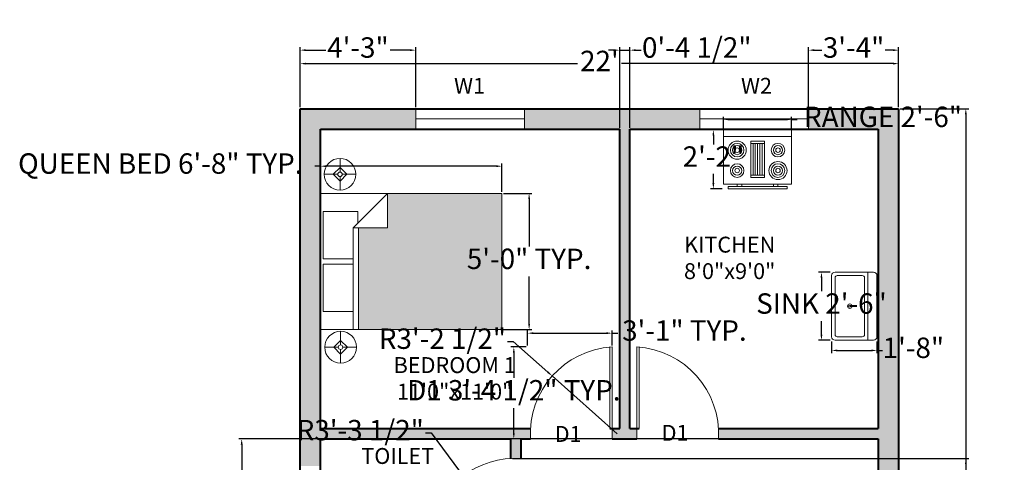
# Model space of a CAD drawing. Units: inches. Extents: x 1883 to 2353, y 1976 to 2541.
# Tile 5 of 5: x 1883 to 2317, y 2346 to 2541. Entities that reach past the tile are written whole.
import ezdxf

# ---------------------------------------------------------------- set-up
doc = ezdxf.new("R2010")
doc.units = ezdxf.units.IN
for name, color, linetype, lineweight in [('A-ANNO-DIMS', 2, 'Continuous', 18), ('A-ANNO-TEXT', 7, 'Continuous', 18), ('A-AREA-IDEN', 7, 'Continuous', 18), ('A-DOOR', 3, 'Continuous', 18), ('A-EQPM', 8, 'Continuous', 18), ('A-FLOR-FIXT', 9, 'Continuous', 18), ('A-FURN', 8, 'Continuous', 18), ('A-GLAZ', 4, 'Continuous', 18), ('A-WALL', 7, 'Continuous', 40)]:
    doc.layers.add(name, color=color, linetype=linetype, lineweight=lineweight)
doc.layers.add('A-FURN-PATT', color=18, linetype='Continuous', lineweight=13, true_color=0x000000)
doc.layers.add('A-WALL-PATT', color=67, linetype='Continuous', lineweight=13, true_color=0x727430)
doc.styles.get("Standard").update_dxf_attribs({"font": 'arial.ttf'})
doc.dimstyles.new('ISO-25', dxfattribs={"dimtxt": 9, "dimasz": 2.5, "dimexe": 1.25, "dimexo": 0.625, "dimgap": 2, "dimtad": 0, "dimtih": 1, "dimtoh": 1, "dimdec": 1, "dimlunit": 4, "dimtxsty": 'Standard', "dimcen": 2.5, "dimadec": 0, "dimazin": 0, "dimtfac": 1, "dimtdec": 1, "dimtmove": 0, "dimatfit": 3, "dimfxl": 1, "dimarcsym": 0})

# ---------------------------------------------------------------- blocks, each defined once
blk = doc.blocks.new('Bed - Queen')
for p, q in [((0, -80.00003), (0, 0)), ((0, 0), (59.99999, 0)), ((59.99999, 0), (59.99999, -80.00003)), ((7.99999, -1.2), (28.79998, -1.2)), ((7.99999, -14.4), (7.99999, -1.2)), ((28.79998, -1.2), (28.79998, -14.4)), ((31.19999, -1.2), (51.99999, -1.2)), ((31.19999, -14.4), (31.19999, -1.2)), ((51.99999, -1.2), (51.99999, -16.4)), ((0, -14.4), (44.8, -14.4)), ((44.8, -16.8), (0, -16.8)), ((59.99999, -29.6), (44.8, -14.4)), ((44.8, -14.4), (44.8, -29.6)), ((51.99999, -16.4), (46.79936, -16.4)), ((44.8, -29.6), (59.99999, -29.6)), ((59.99999, -80.00003), (0, -80.00003))]:
    blk.add_line(p, q)
blk = doc.blocks.new('Range-Oven - 30 in top')
for p, q in [((0, -3), (30, -3)), ((12, -6), (18, -6)), ((13, -20), (13, -6)), ((14, -6), (14, -20)), ((15, -20), (15, -6)), ((16, -6), (16, -20)), ((17, -20), (17, -6)), ((18, -20), (12, -20)), ((6, -24), (6, -25)), ((8, -25), (8, -24)), ((22, -25), (22, -24)), ((24, -24), (24, -25))]:
    blk.add_line(p, q)
for points in [[(0, -24), (0, 0), (30, 0), (30, -24)], [(12, -21), (12, -5), (18, -5), (18, -21)], [(2, -26), (2, -25), (28, -25), (28, -26)]]:
    blk.add_lwpolyline(points, close=True)
for centre, radius in [((6, -9), 4), ((6, -9), 3), ((6, -9), 2), ((6, -9), 1), ((24, -9), 3), ((24, -9), 2), ((24, -9), 1), ((6, -18), 3), ((6, -18), 2), ((6, -18), 1), ((24, -18), 4), ((24, -18), 3), ((24, -18), 2), ((24, -18), 1)]:
    blk.add_circle(centre, radius)
blk = doc.blocks.new('Sink-single - 30 in top')
blk.add_line((-15, -3.999996), (15, -3.999996))
for points in [[(-13.5, 0), (13.5, 0)], [(-15, -18.499996), (-15, -1.5)], [(15, -1.5), (15, -18.499996)], [(-13.5, -17.499996), (-13.5, -6.499996)], [(-12.5, -5.499996), (12.5, -5.499996)], [(13.5, -6.499996), (13.5, -17.499996)], [(13.5, -19.999996), (-13.5, -19.999996)], [(12.5, -18.499996), (-12.5, -18.499996)]]:
    blk.add_lwpolyline(points)
for radius in [1, 0.5]:
    blk.add_circle((0, -11.999996), radius)
for centre, radius, start, end in [((-13.5, -1.5), 1.5, 90, 180), ((13.5, -1.5), 1.5, 0, 90), ((-12.5, -6.499996), 1, 90, 180), ((12.5, -6.499996), 1, 0, 90), ((-13.5, -18.499996), 1.5, 180, 270), ((-12.5, -17.499996), 1, 180, 270), ((12.5, -17.499996), 1, 270, 0), ((13.5, -18.499996), 1.5, 270, 0)]:
    blk.add_arc(centre, radius, start, end)
blk = doc.blocks.new('Lamp - Table')
for p, q in [((0, 7), (0, 1)), ((-1, 0), (-7, 0)), ((0, 3), (-3, 0)), ((-3, 0), (0, -3)), ((3, 0), (0, 3)), ((0, -3), (3, 0)), ((1, 0), (7, 0)), ((0, -1), (0, -7))]:
    blk.add_line(p, q)
for radius in [7, 1]:
    blk.add_circle((0, 0), radius)
blk = doc.blocks.new('*D15')
at = {"layer": 'A-ANNO-DIMS', "color": 0, "lineweight": -2, "transparency": 16777216}
for p, q in [((2006.49, 2502.7), (2006.49, 2523.19)), ((2008.99, 2521.94), (2128.78, 2521.94)), ((2267.99, 2521.94), (2148.21, 2521.94)), ((2270.49, 2502.7), (2270.49, 2523.19))]:
    blk.add_line(p, q, dxfattribs=at)
at = {"layer": 'A-ANNO-DIMS', "color": 0, "transparency": 16777216}
for points in [[(2008.99, 2522.36), (2008.99, 2521.53), (2006.49, 2521.94)], [(2267.99, 2522.36), (2267.99, 2521.53), (2270.49, 2521.94)]]:
    blk.add_solid(points, dxfattribs=at)
at = {"layer": 'Defpoints', "color": 0, "transparency": 16777216}
for p in [(2270.49, 2521.94), (2006.49, 2502.07), (2270.49, 2502.07)]:
    blk.add_point(p, dxfattribs=at)
at = {"layer": 'A-ANNO-DIMS', "color": 0, "transparency": 16777216, "insert": (2138.49, 2521.94), "char_height": 9, "attachment_point": 5}
blk.add_mtext("22'", dxfattribs=at)
blk = doc.blocks.new('WIN-48IN')
for p, q in [((0, 0), (0, 9)), ((48, 0), (48, 9)), ((0, 4.5), (48, 4.5))]:
    blk.add_line(p, q)
blk = doc.blocks.new('DOOR-SWING-36IN')
for p, q in [((35.07, 4.5), (35.07, 40.5)), ((36.07, 4.5), (36.07, 40.5)), ((0.07, 4.5), (0.07, 0)), ((36.07, 4.5), (36.07, 0))]:
    blk.add_line(p, q)
blk.add_arc((38.32, 2.25), 38.32, 93.3665, 183.3665)
blk = doc.blocks.new('*D25')
at = {"layer": 'A-ANNO-DIMS', "color": 0, "lineweight": -2, "transparency": 16777216}
for p, q in [((2015.49, 2476.74), (2012.99, 2476.74)), ((2015.49, 2465.37), (2015.49, 2477.99)), ((2092.99, 2476.74), (2017.99, 2476.74)), ((2095.49, 2465.37), (2095.49, 2477.99))]:
    blk.add_line(p, q, dxfattribs=at)
at = {"layer": 'A-ANNO-DIMS', "color": 0, "transparency": 16777216}
for points in [[(2017.99, 2477.16), (2017.99, 2476.33), (2015.49, 2476.74)], [(2092.99, 2477.16), (2092.99, 2476.33), (2095.49, 2476.74)]]:
    blk.add_solid(points, dxfattribs=at)
at = {"layer": 'Defpoints', "color": 0, "transparency": 16777216}
for p in [(2015.49, 2476.74), (2015.49, 2464.74), (2095.49, 2464.74)]:
    blk.add_point(p, dxfattribs=at)
at = {"layer": 'A-ANNO-DIMS', "color": 0, "transparency": 16777216, "insert": (1944.8, 2476.74), "char_height": 9, "attachment_point": 5}
blk.add_mtext('QUEEN BED 6\'-8" TYP.', dxfattribs=at)
blk = doc.blocks.new('*D26')
at = {"layer": 'A-ANNO-DIMS', "color": 0, "lineweight": -2, "transparency": 16777216}
for p, q in [((2096.12, 2464.74), (2108.74, 2464.74)), ((2107.49, 2462.24), (2107.49, 2441.34)), ((2107.49, 2407.24), (2107.49, 2428.15)), ((2096.12, 2404.74), (2108.74, 2404.74))]:
    blk.add_line(p, q, dxfattribs=at)
at = {"layer": 'A-ANNO-DIMS', "color": 0, "transparency": 16777216}
for points in [[(2107.08, 2462.24), (2107.91, 2462.24), (2107.49, 2464.74)], [(2107.08, 2407.24), (2107.91, 2407.24), (2107.49, 2404.74)]]:
    blk.add_solid(points, dxfattribs=at)
at = {"layer": 'Defpoints', "color": 0, "transparency": 16777216}
for p in [(2095.49, 2464.74), (2107.49, 2464.74), (2095.49, 2404.74)]:
    blk.add_point(p, dxfattribs=at)
at = {"layer": 'A-ANNO-DIMS', "color": 0, "transparency": 16777216, "insert": (2107.49, 2434.74), "char_height": 9, "attachment_point": 5}
blk.add_mtext('5\'-0" TYP.', dxfattribs=at)
blk = doc.blocks.new('*D29')
at = {"layer": 'A-ANNO-DIMS', "color": 0, "lineweight": -2, "transparency": 16777216}
for p, q in [((2106.19, 2397.07), (2099.49, 2397.07)), ((2100.74, 2394.57), (2100.74, 2383.48)), ((2100.74, 2359.07), (2100.74, 2370.17)), ((2106.19, 2356.57), (2099.49, 2356.57))]:
    blk.add_line(p, q, dxfattribs=at)
at = {"layer": 'A-ANNO-DIMS', "color": 0, "transparency": 16777216}
for points in [[(2100.33, 2394.57), (2101.16, 2394.57), (2100.74, 2397.07)], [(2100.33, 2359.07), (2101.16, 2359.07), (2100.74, 2356.57)]]:
    blk.add_solid(points, dxfattribs=at)
at = {"layer": 'Defpoints', "color": 0, "transparency": 16777216}
for p in [(2100.74, 2397.07), (2106.82, 2397.07), (2106.82, 2356.57)]:
    blk.add_point(p, dxfattribs=at)
at = {"layer": 'A-ANNO-DIMS', "color": 0, "transparency": 16777216, "insert": (2100.74, 2376.82), "char_height": 9, "attachment_point": 5}
blk.add_mtext('D1 3\'-4 1/2" TYP.', dxfattribs=at)
blk = doc.blocks.new('*D30')
at = {"layer": 'A-ANNO-DIMS', "color": 0, "lineweight": -2, "transparency": 16777216}
for p, q in [((2106.82, 2397.7), (2106.82, 2404.4)), ((2109.32, 2403.15), (2141.56, 2403.15)), ((2144.06, 2397.7), (2144.06, 2404.4)), ((2144.06, 2403.15), (2146.56, 2403.15))]:
    blk.add_line(p, q, dxfattribs=at)
at = {"layer": 'A-ANNO-DIMS', "color": 0, "transparency": 16777216}
for points in [[(2109.32, 2403.56), (2109.32, 2402.73), (2106.82, 2403.15)], [(2141.56, 2403.56), (2141.56, 2402.73), (2144.06, 2403.15)]]:
    blk.add_solid(points, dxfattribs=at)
at = {"layer": 'Defpoints', "color": 0, "transparency": 16777216}
for p in [(2144.06, 2403.15), (2106.82, 2397.07), (2144.06, 2397.07)]:
    blk.add_point(p, dxfattribs=at)
at = {"layer": 'A-ANNO-DIMS', "color": 0, "transparency": 16777216, "insert": (2175.99, 2403.15), "char_height": 9, "attachment_point": 5}
blk.add_mtext('3\'-1" TYP.', dxfattribs=at)
blk = doc.blocks.new('*D39')
at = {"layer": 'A-ANNO-DIMS', "color": 0, "lineweight": -2, "transparency": 16777216}
for p, q in [((2193.27, 2493.44), (2193.27, 2498.56)), ((2223.27, 2493.44), (2223.27, 2498.56)), ((2195.77, 2497.31), (2220.77, 2497.31)), ((2223.27, 2497.31), (2225.77, 2497.31))]:
    blk.add_line(p, q, dxfattribs=at)
at = {"layer": 'A-ANNO-DIMS', "color": 0, "transparency": 16777216}
for points in [[(2195.77, 2497.73), (2195.77, 2496.9), (2193.27, 2497.31)], [(2220.77, 2497.73), (2220.77, 2496.9), (2223.27, 2497.31)]]:
    blk.add_solid(points, dxfattribs=at)
at = {"layer": 'Defpoints', "color": 0, "transparency": 16777216}
for p in [(2223.27, 2497.31), (2193.27, 2492.81), (2223.27, 2492.81)]:
    blk.add_point(p, dxfattribs=at)
at = {"layer": 'A-ANNO-DIMS', "color": 0, "transparency": 16777216, "insert": (2263.6, 2497.31), "char_height": 9, "attachment_point": 5}
blk.add_mtext('RANGE 2\'-6"', dxfattribs=at)
blk = doc.blocks.new('*D40')
at = {"layer": 'A-ANNO-DIMS', "color": 0, "lineweight": -2, "transparency": 16777216}
for p, q in [((2192.64, 2492.81), (2187.52, 2492.81)), ((2188.77, 2490.31), (2188.77, 2486.33)), ((2188.77, 2469.31), (2188.77, 2473.3)), ((2192.64, 2466.81), (2187.52, 2466.81))]:
    blk.add_line(p, q, dxfattribs=at)
at = {"layer": 'A-ANNO-DIMS', "color": 0, "transparency": 16777216}
for points in [[(2188.35, 2490.31), (2189.18, 2490.31), (2188.77, 2492.81)], [(2188.35, 2469.31), (2189.18, 2469.31), (2188.77, 2466.81)]]:
    blk.add_solid(points, dxfattribs=at)
at = {"layer": 'Defpoints', "color": 0, "transparency": 16777216}
for p in [(2188.77, 2492.81), (2193.27, 2492.81), (2193.27, 2466.81)]:
    blk.add_point(p, dxfattribs=at)
at = {"layer": 'A-ANNO-DIMS', "color": 0, "transparency": 16777216, "insert": (2188.77, 2479.81), "char_height": 9, "attachment_point": 5}
blk.add_mtext('2\'-2"', dxfattribs=at)
blk = doc.blocks.new('*D41')
at = {"layer": 'A-ANNO-DIMS', "color": 0, "lineweight": -2, "transparency": 16777216}
for p, q in [((2240.32, 2430.04), (2235.2, 2430.04)), ((2236.45, 2427.54), (2236.45, 2421.69)), ((2236.45, 2402.54), (2236.45, 2408.39)), ((2240.32, 2400.04), (2235.2, 2400.04))]:
    blk.add_line(p, q, dxfattribs=at)
at = {"layer": 'A-ANNO-DIMS', "color": 0, "transparency": 16777216}
for points in [[(2236.03, 2427.54), (2236.86, 2427.54), (2236.45, 2430.04)], [(2236.03, 2402.54), (2236.86, 2402.54), (2236.45, 2400.04)]]:
    blk.add_solid(points, dxfattribs=at)
at = {"layer": 'Defpoints', "color": 0, "transparency": 16777216}
for p in [(2240.95, 2430.04), (2236.45, 2400.04), (2240.95, 2400.04)]:
    blk.add_point(p, dxfattribs=at)
at = {"layer": 'A-ANNO-DIMS', "color": 0, "transparency": 16777216, "insert": (2236.45, 2415.04), "char_height": 9, "attachment_point": 5}
blk.add_mtext('SINK 2\'-6"', dxfattribs=at)
blk = doc.blocks.new('*D42')
at = {"layer": 'A-ANNO-DIMS', "color": 0, "lineweight": -2, "transparency": 16777216}
for p, q in [((2240.95, 2399.41), (2240.95, 2394.29)), ((2260.95, 2399.41), (2260.95, 2394.29)), ((2243.45, 2395.54), (2258.45, 2395.54)), ((2260.95, 2395.54), (2263.45, 2395.54))]:
    blk.add_line(p, q, dxfattribs=at)
at = {"layer": 'A-ANNO-DIMS', "color": 0, "transparency": 16777216}
for points in [[(2243.45, 2395.96), (2243.45, 2395.12), (2240.95, 2395.54)], [(2258.45, 2395.96), (2258.45, 2395.12), (2260.95, 2395.54)]]:
    blk.add_solid(points, dxfattribs=at)
at = {"layer": 'Defpoints', "color": 0, "transparency": 16777216}
for p in [(2240.95, 2400.04), (2260.95, 2400.04), (2260.95, 2395.54)]:
    blk.add_point(p, dxfattribs=at)
at = {"layer": 'A-ANNO-DIMS', "color": 0, "transparency": 16777216, "insert": (2276.99, 2395.54), "char_height": 9, "attachment_point": 5}
blk.add_mtext('1\'-8"', dxfattribs=at)
blk = doc.blocks.new('*D43')
at = {"layer": 'A-ANNO-DIMS', "color": 0, "lineweight": -2, "transparency": 16777216}
for p, q in [((2271.12, 2502.07), (2301.39, 2502.07)), ((2300.14, 2499.57), (2300.14, 2267.17)), ((2300.14, 2021.57), (2300.14, 2253.97)), ((2271.12, 2019.07), (2301.39, 2019.07))]:
    blk.add_line(p, q, dxfattribs=at)
at = {"layer": 'A-ANNO-DIMS', "color": 0, "transparency": 16777216}
for points in [[(2299.73, 2499.57), (2300.56, 2499.57), (2300.14, 2502.07)], [(2299.73, 2021.57), (2300.56, 2021.57), (2300.14, 2019.07)]]:
    blk.add_solid(points, dxfattribs=at)
at = {"layer": 'Defpoints', "color": 0, "transparency": 16777216}
for p in [(2270.49, 2502.07), (2300.14, 2502.07), (2270.49, 2019.07)]:
    blk.add_point(p, dxfattribs=at)
at = {"layer": 'A-ANNO-DIMS', "color": 0, "transparency": 16777216, "insert": (2300.14, 2260.57), "char_height": 9, "attachment_point": 5}
blk.add_mtext('40\'-3"', dxfattribs=at)
blk = doc.blocks.new('*D48')
at = {"layer": 'A-ANNO-DIMS', "color": 0, "lineweight": -2, "transparency": 16777216}
for p, q in [((2260.87, 2356.57), (1979.44, 2356.57)), ((1980.69, 2354.07), (1980.69, 2342.73)), ((1980.69, 2318.19), (1980.69, 2329.53)), ((2260.87, 2315.69), (1979.44, 2315.69))]:
    blk.add_line(p, q, dxfattribs=at)
at = {"layer": 'A-ANNO-DIMS', "color": 0, "transparency": 16777216}
for points in [[(1980.28, 2354.07), (1981.11, 2354.07), (1980.69, 2356.57)], [(1980.28, 2318.19), (1981.11, 2318.19), (1980.69, 2315.69)]]:
    blk.add_solid(points, dxfattribs=at)
at = {"layer": 'Defpoints', "color": 0, "transparency": 16777216}
for p in [(1980.69, 2356.57), (2261.49, 2356.57), (2261.49, 2315.69)]:
    blk.add_point(p, dxfattribs=at)
at = {"layer": 'A-ANNO-DIMS', "color": 0, "transparency": 16777216, "insert": (1980.69, 2336.13), "char_height": 9, "attachment_point": 5}
blk.add_mtext('3\'-5"', dxfattribs=at)
blk = doc.blocks.new('*D49')
at = {"layer": 'A-ANNO-DIMS', "color": 0, "lineweight": -2, "transparency": 16777216}
for p, q in [((2006.49, 2502.7), (2006.49, 2529.12)), ((2057.49, 2502.7), (2057.49, 2529.12)), ((2008.99, 2527.87), (2017.85, 2527.87)), ((2054.99, 2527.87), (2046.14, 2527.87))]:
    blk.add_line(p, q, dxfattribs=at)
at = {"layer": 'A-ANNO-DIMS', "color": 0, "transparency": 16777216}
for points in [[(2008.99, 2528.29), (2008.99, 2527.46), (2006.49, 2527.87)], [(2054.99, 2528.29), (2054.99, 2527.46), (2057.49, 2527.87)]]:
    blk.add_solid(points, dxfattribs=at)
at = {"layer": 'Defpoints', "color": 0, "transparency": 16777216}
for p in [(2057.49, 2527.87), (2006.49, 2502.07), (2057.49, 2502.07)]:
    blk.add_point(p, dxfattribs=at)
at = {"layer": 'A-ANNO-DIMS', "color": 0, "transparency": 16777216, "insert": (2031.99, 2527.87), "char_height": 9, "attachment_point": 5}
blk.add_mtext('4\'-3"', dxfattribs=at)
blk = doc.blocks.new('*D50')
at = {"layer": 'A-ANNO-DIMS', "color": 0, "lineweight": -2, "transparency": 16777216}
for p, q in [((2230.74, 2502.7), (2230.74, 2529.12)), ((2270.49, 2502.7), (2270.49, 2529.12)), ((2233.24, 2527.87), (2236.66, 2527.87)), ((2267.99, 2527.87), (2264.58, 2527.87))]:
    blk.add_line(p, q, dxfattribs=at)
at = {"layer": 'A-ANNO-DIMS', "color": 0, "transparency": 16777216}
for points in [[(2233.24, 2528.29), (2233.24, 2527.46), (2230.74, 2527.87)], [(2267.99, 2528.29), (2267.99, 2527.46), (2270.49, 2527.87)]]:
    blk.add_solid(points, dxfattribs=at)
at = {"layer": 'Defpoints', "color": 0, "transparency": 16777216}
for p in [(2270.49, 2527.87), (2230.74, 2502.07), (2270.49, 2502.07)]:
    blk.add_point(p, dxfattribs=at)
at = {"layer": 'A-ANNO-DIMS', "color": 0, "transparency": 16777216, "insert": (2250.62, 2527.87), "char_height": 9, "attachment_point": 5}
blk.add_mtext('3\'-4"', dxfattribs=at)
blk = doc.blocks.new('*D54')
at = {"layer": 'A-ANNO-DIMS', "color": 0, "lineweight": -2, "transparency": 16777216}
for p, q in [((2100.12, 2347.93), (2301.39, 2347.93)), ((2300.14, 2345.43), (2300.14, 2339.52)), ((2300.14, 2320.43), (2300.14, 2326.33)), ((2100.12, 2317.93), (2301.39, 2317.93))]:
    blk.add_line(p, q, dxfattribs=at)
at = {"layer": 'A-ANNO-DIMS', "color": 0, "transparency": 16777216}
for points in [[(2299.73, 2345.43), (2300.56, 2345.43), (2300.14, 2347.93)], [(2299.73, 2320.43), (2300.56, 2320.43), (2300.14, 2317.93)]]:
    blk.add_solid(points, dxfattribs=at)
at = {"layer": 'Defpoints', "color": 0, "transparency": 16777216}
for p in [(2099.49, 2347.93), (2300.14, 2347.93), (2099.49, 2317.93)]:
    blk.add_point(p, dxfattribs=at)
at = {"layer": 'A-ANNO-DIMS', "color": 0, "transparency": 16777216, "insert": (2300.14, 2332.93), "char_height": 9, "attachment_point": 5}
blk.add_mtext('2\'-6"', dxfattribs=at)
blk = doc.blocks.new('*D58')
at = {"layer": 'A-ANNO-DIMS', "color": 0, "lineweight": -2, "transparency": 16777216}
for p, q in [((2147.49, 2493.7), (2147.49, 2529.12)), ((2151.99, 2493.7), (2151.99, 2529.12)), ((2144.99, 2527.87), (2142.49, 2527.87)), ((2147.49, 2527.87), (2151.99, 2527.87)), ((2154.49, 2527.87), (2156.99, 2527.87))]:
    blk.add_line(p, q, dxfattribs=at)
at = {"layer": 'A-ANNO-DIMS', "color": 0, "transparency": 16777216}
for points in [[(2144.99, 2528.29), (2144.99, 2527.46), (2147.49, 2527.87)], [(2154.49, 2528.29), (2154.49, 2527.46), (2151.99, 2527.87)]]:
    blk.add_solid(points, dxfattribs=at)
at = {"layer": 'Defpoints', "color": 0, "transparency": 16777216}
for p in [(2151.99, 2527.87), (2147.49, 2493.07), (2151.99, 2493.07)]:
    blk.add_point(p, dxfattribs=at)
at = {"layer": 'A-ANNO-DIMS', "color": 0, "transparency": 16777216, "insert": (2181.44, 2527.87), "char_height": 9, "attachment_point": 5}
blk.add_mtext('0\'-4 1/2"', dxfattribs=at)
blk = doc.blocks.new('*D60')
at = {"layer": 'A-ANNO-DIMS', "color": 0, "lineweight": -2, "transparency": 16777216}
for p, q in [((2061.75, 2359.24), (2064.25, 2359.24)), ((2064.25, 2359.24), (2076.82, 2342.27)), ((2101.74, 2308.63), (2078.31, 2340.26))]:
    blk.add_line(p, q, dxfattribs=at)
at = {"layer": 'A-ANNO-DIMS', "color": 0, "transparency": 16777216}
blk.add_solid([(2077.16, 2342.51), (2076.49, 2342.02), (2078.31, 2340.26)], dxfattribs=at)
at = {"layer": 'Defpoints', "color": 0, "transparency": 16777216}
for p in [(2078.31, 2340.26), (2101.74, 2308.63)]:
    blk.add_point(p, dxfattribs=at)
at = {"layer": 'A-ANNO-DIMS', "color": 0, "transparency": 16777216, "insert": (2033, 2359.24), "char_height": 9, "attachment_point": 5}
blk.add_mtext('R3\'-3 1/2"', dxfattribs=at)
blk = doc.blocks.new('*D63')
at = {"layer": 'A-ANNO-DIMS', "color": 0, "lineweight": -2, "transparency": 16777216}
for p, q in [((2097.99, 2399.55), (2100.49, 2399.55)), ((2100.49, 2399.55), (2115.81, 2385.94)), ((2146.31, 2358.82), (2117.67, 2384.28))]:
    blk.add_line(p, q, dxfattribs=at)
at = {"layer": 'A-ANNO-DIMS', "color": 0, "transparency": 16777216}
blk.add_solid([(2116.08, 2386.25), (2115.53, 2385.63), (2117.67, 2384.28)], dxfattribs=at)
at = {"layer": 'Defpoints', "color": 0, "transparency": 16777216}
for p in [(2117.67, 2384.28), (2146.31, 2358.82)]:
    blk.add_point(p, dxfattribs=at)
at = {"layer": 'A-ANNO-DIMS', "color": 0, "transparency": 16777216, "insert": (2069.24, 2399.55), "char_height": 9, "attachment_point": 5}
blk.add_mtext('R3\'-2 1/2"', dxfattribs=at)

msp = doc.modelspace()

# ---------------------------------------------------------------- hatches: boundary and pattern name
at = {"layer": 'A-FURN-PATT'}
h = msp.add_hatch(color=256, dxfattribs=at)
h.dxf.hatch_style = 1
h.paths.add_polyline_path([(2095.49, 2464.74), (2045.09, 2464.74), (2045.09, 2449.54), (2032.29, 2449.54), (2032.29, 2404.74), (2095.49, 2404.74)])
h.paths.add_polyline_path([(2095.49, 2201.04), (2045.09, 2201.04), (2045.09, 2185.84), (2032.29, 2185.84), (2032.29, 2141.04), (2095.49, 2141.04)])
at = {"layer": 'A-WALL-PATT'}
h = msp.add_hatch(color=256, dxfattribs=at)
h.dxf.hatch_style = 1
h.paths.add_polyline_path([(2057.49, 2502.07), (2006.49, 2502.07), (2006.49, 2344.57), (2015.49, 2344.57), (2015.49, 2356.57), (2099.49, 2356.57), (2099.49, 2347.93), (2103.99, 2347.93), (2103.99, 2356.57), (2108.06, 2356.57, -0.029386), (2108.06, 2361.07), (2015.49, 2361.07), (2015.49, 2493.07), (2057.49, 2493.07)])
h.paths.add_polyline_path([(2182.74, 2502.07), (2105.49, 2502.07), (2105.49, 2493.07), (2147.49, 2493.07), (2147.49, 2361.07), (2144.06, 2361.07), (2144.06, 2356.57), (2151.99, 2356.57), (2155, 2356.57), (2155, 2361.07), (2151.99, 2361.07), (2151.99, 2493.07), (2182.74, 2493.07)])
h.paths.add_polyline_path([(2270.49, 2502.07), (2230.74, 2502.07), (2230.74, 2493.07), (2261.49, 2493.07), (2261.49, 2361.07), (2191, 2361.07, -0.029386), (2191, 2356.57), (2261.49, 2356.57), (2261.49, 2315.69), (2270.49, 2315.69)])
h.paths.add_polyline_path([(2051.49, 2131.57), (2015.49, 2131.57), (2015.49, 2251.57), (2103.99, 2251.57), (2104.81, 2251.57, -0.028441), (2104.81, 2256.07), (2103.99, 2256.07), (2103.99, 2260.88), (2099.49, 2260.88), (2099.49, 2256.07), (2015.49, 2256.07), (2015.49, 2268.07), (2006.49, 2268.07), (2006.49, 2122.57), (2015.49, 2122.57), (2051.49, 2122.57)])
h.paths.add_polyline_path([(2103.99, 2308.57), (2103.99, 2317.93, -0.034841), (2099.49, 2317.93), (2099.49, 2308.57), (2015.49, 2308.57), (2015.49, 2320.57), (2006.49, 2320.57), (2006.49, 2292.07), (2015.49, 2292.07), (2015.49, 2304.07), (2099.49, 2304.07), (2099.49, 2290.88, -0.034841), (2103.99, 2290.88), (2103.99, 2304.07)])

# ---------------------------------------------------------------- linework, layer by layer
at = {"layer": 'A-DOOR'}
msp.add_arc((2101.74, 2308.63), 39.36, 86.7233, 166.3344, dxfattribs=at)
at = {"layer": 'A-WALL'}
for p, q in [((2006.49, 2502.07), (2270.49, 2502.07)), ((2006.49, 2122.57), (2006.49, 2502.07)), ((2270.49, 2502.07), (2270.49, 2094.07)), ((2015.49, 2493.07), (2147.49, 2493.07)), ((2015.49, 2361.07), (2015.49, 2493.07)), ((2147.49, 2361.07), (2147.49, 2493.07)), ((2151.99, 2361.07), (2151.99, 2493.07)), ((2151.99, 2493.07), (2261.49, 2493.07)), ((2261.49, 2493.07), (2261.49, 2361.07)), ((2015.49, 2361.07), (2108.06, 2361.07)), ((2143.06, 2361.07), (2147.49, 2361.07)), ((2151.99, 2361.07), (2156, 2361.07)), ((2191, 2361.07), (2261.49, 2361.07)), ((2015.49, 2356.57), (2099.49, 2356.57)), ((2015.49, 2308.57), (2015.49, 2356.57)), ((2099.49, 2347.93), (2099.49, 2356.57)), ((2103.99, 2356.57), (2108.06, 2356.57)), ((2103.99, 2347.93), (2103.99, 2356.57)), ((2144.06, 2356.57), (2151.99, 2356.57)), ((2151.99, 2356.57), (2155, 2356.57)), ((2191, 2356.57), (2261.49, 2356.57)), ((2261.49, 2356.57), (2261.49, 2200.57))]:
    msp.add_line(p, q, dxfattribs=at)

# ---------------------------------------------------------------- block references
at = {"layer": 'A-DOOR'}
msp.add_blockref('DOOR-SWING-36IN', (2108, 2356.57), dxfattribs=at)
at = {"layer": 'A-DOOR', "extrusion": (0, 0, -1), "zscale": -1}
msp.add_blockref('DOOR-SWING-36IN', (-2191.06, 2356.57), dxfattribs=at)
at = {"layer": 'A-EQPM'}
msp.add_blockref('Range-Oven - 30 in top', (2193.27, 2492.81), dxfattribs=at)
at = {"layer": 'A-FLOR-FIXT', "rotation": 270}
msp.add_blockref('Sink-single - 30 in top', (2260.95, 2415.04), dxfattribs=at)
at = {"layer": 'A-FURN'}
for p in [(2024.07, 2473.17), (2024.32, 2396.97)]:
    msp.add_blockref('Lamp - Table', p, dxfattribs=at)
at = {"layer": 'A-FURN', "rotation": 90}
msp.add_blockref('Bed - Queen', (2015.49, 2404.74), dxfattribs=at)
at = {"layer": 'A-GLAZ'}
for p in [(2057.49, 2493.07), (2182.74, 2493.07)]:
    msp.add_blockref('WIN-48IN', p, dxfattribs=at)

# ---------------------------------------------------------------- texts
at = {"layer": 'A-ANNO-TEXT', "char_height": 7, "attachment_point": 1}
for s, width, insert in [('\\pxqc;{\\fArial|b1|i0|c0|p34;W1}', 23.5361, (2069.45, 2515.66)), ('\\pxqc;{\\fArial|b1|i0|c0|p34;W2}', 23.5361, (2196.02, 2515.66)), ('\\pxqc;{\\fArial|b1|i0|c0|p34;D1}', 15.7077, (2116.84, 2362.24)), ('\\pxqc;{\\fArial|b1|i0|c0|p34;D1}', 15.7077, (2164.03, 2362.72))]:
    msp.add_mtext_dynamic_manual_height_columns(s, width=width, gutter_width=12.5, heights=[0], dxfattribs=dict(at, insert=insert))
at = {"layer": 'A-AREA-IDEN', "char_height": 7, "attachment_point": 1}
for s, width, insert in [('\\pxqc;{\\fArial|b1|i0|c0|p34;KITCHEN\\P8\'0"x9\'0"}', 69.6451, (2161.14, 2445.66)), ('\\pxqc;{\\fArial|b1|i0|c0|p34;BEDROOM 1\\P11\'0"x11\'0"}', 70.2184, (2039.56, 2392.58)), ('\\pxqc;{\\fArial|b1|i0|c0|p34;TOILET\\P4\'0"x7\'0"}', 65.0789, (2017, 2352.53))]:
    msp.add_mtext_dynamic_manual_height_columns(s, width=width, gutter_width=12.5, heights=[0], dxfattribs=dict(at, insert=insert))

# ---------------------------------------------------------------- dimensions: what is measured, and where the dimension line sits
at = {"layer": 'A-ANNO-DIMS'}
for base, p1, p2, override, picture, middle in [((2151.99, 2527.87), (2147.49, 2493.07), (2151.99, 2493.07), {"dimdec": 1, "dimlfac": 1, "dimrnd": 0, "dimzin": 1, "dimdsep": 46, "dimlunit": 4, "dimfrac": 2}, '*D58', (2181.44, 2527.87)), ((2057.49, 2527.87), (2006.49, 2502.07), (2057.49, 2502.07), {"dimdec": 1, "dimlfac": 1, "dimrnd": 0, "dimzin": 1, "dimdsep": 46, "dimlunit": 4, "dimfrac": 2}, '*D49', (2031.99, 2527.87)), ((2270.493684, 2527.871955), (2230.743684, 2502.071955), (2270.493684, 2502.071955), {"dimdec": 1, "dimlfac": 1, "dimrnd": 0, "dimzin": 1, "dimdsep": 46, "dimlunit": 4, "dimfrac": 2}, '*D50', (2250.618684, 2527.871955)), ((2270.49, 2521.94), (2006.49, 2502.07), (2270.49, 2502.07), {"dimclrd": 0, "dimclre": 0, "dimclrt": 0}, '*D15', (2138.49, 2521.94)), ((2260.95, 2395.54), (2240.95, 2400.04), (2260.95, 2400.04), {"dimdec": 1, "dimlfac": 1, "dimrnd": 0, "dimzin": 1, "dimdsep": 46, "dimlunit": 4, "dimfrac": 2}, '*D42', (2276.99, 2395.54))]:
    dim = msp.add_linear_dim(base=base, p1=p1, p2=p2, dimstyle='ISO-25', override=override, dxfattribs=at)
    dim.commit()
    dim.dimension.update_dxf_attribs({"geometry": picture, "text_midpoint": middle})
for base, p1, p2, text, picture, middle in [((2223.27, 2497.31), (2193.27, 2492.81), (2223.27, 2492.81), 'RANGE <>', '*D39', (2263.6, 2497.31)), ((2144.06, 2403.15), (2106.82, 2397.07), (2144.06, 2397.07), '<> TYP.', '*D30', (2175.99, 2403.15))]:
    dim = msp.add_linear_dim(base=base, p1=p1, p2=p2, text=text, dimstyle='ISO-25', override={"dimdec": 1, "dimlfac": 1, "dimrnd": 0, "dimzin": 1, "dimdsep": 46, "dimlunit": 4, "dimfrac": 2}, dxfattribs=at)
    dim.commit()
    dim.dimension.update_dxf_attribs({"geometry": picture, "text_midpoint": middle})
for base, p1, p2, angle, text, picture, middle in [((2015.49, 2476.74), (2095.49, 2464.74), (2015.49, 2464.74), 180, 'QUEEN BED <> TYP.', '*D25', (1944.8, 2476.74)), ((2107.49, 2464.74), (2095.49, 2404.74), (2095.49, 2464.74), 90, '<> TYP.', '*D26', (2107.49, 2434.74)), ((2236.45, 2400.04), (2240.95, 2430.04), (2240.95, 2400.04), 270, 'SINK <>', '*D41', (2236.45, 2415.04)), ((2100.74, 2397.07), (2106.82, 2356.57), (2106.82, 2397.07), 90, 'D1 <> TYP.', '*D29', (2100.74, 2376.82))]:
    dim = msp.add_linear_dim(base=base, p1=p1, p2=p2, angle=angle, text=text, dimstyle='ISO-25', override={"dimdec": 1, "dimlfac": 1, "dimrnd": 0, "dimzin": 1, "dimdsep": 46, "dimlunit": 4, "dimfrac": 2}, dxfattribs=at)
    dim.commit()
    dim.dimension.update_dxf_attribs({"geometry": picture, "text_midpoint": middle})
for base, p1, p2, picture, middle in [((2300.14, 2502.07), (2270.49, 2019.07), (2270.49, 2502.07), '*D43', (2300.14, 2260.57)), ((2188.77, 2492.81), (2193.27, 2466.81), (2193.27, 2492.81), '*D40', (2188.77, 2479.81)), ((1980.69, 2356.57), (2261.49, 2315.69), (2261.49, 2356.57), '*D48', (1980.69, 2336.13)), ((2300.14, 2347.93), (2099.49, 2317.93), (2099.49, 2347.93), '*D54', (2300.14, 2332.93))]:
    dim = msp.add_linear_dim(base=base, p1=p1, p2=p2, angle=90, dimstyle='ISO-25', override={"dimdec": 1, "dimlfac": 1, "dimrnd": 0, "dimzin": 1, "dimdsep": 46, "dimlunit": 4, "dimfrac": 2}, dxfattribs=at)
    dim.commit()
    dim.dimension.update_dxf_attribs({"geometry": picture, "text_midpoint": middle})
for center, mpoint, picture, middle in [((2146.31, 2358.82), (2117.67, 2384.28), '*D63', (2069.24, 2399.55)), ((2101.74, 2308.63), (2078.31, 2340.26), '*D60', (2033, 2359.24))]:
    dim = msp.add_radius_dim(center=center, mpoint=mpoint, dimstyle='ISO-25', override={"dimdec": 1, "dimlfac": 1, "dimrnd": 0, "dimzin": 1, "dimdsep": 46, "dimlunit": 4, "dimfrac": 2}, dxfattribs=at)
    dim.commit()
    dim.dimension.update_dxf_attribs({"geometry": picture, "text_midpoint": middle, "dimtype": 164})

doc.saveas('drawing.dxf')
